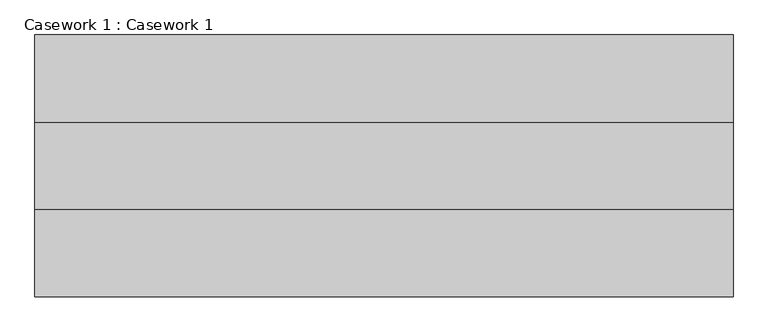
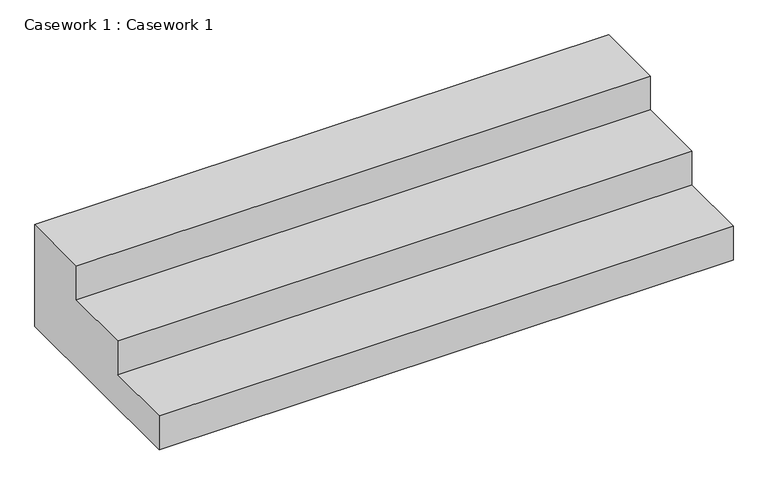
"""IFC4 building model written with IfcOpenShell, lengths in millimetres: furniture geometry, Casework 1 : Casework 1."""

from ifc_helpers import new_model, si_unit, frame, origin, place, context, project, spatial, polyline, outline, extrude, source, transform, mapped, element, save


def casework_1_casework_1_59e189ff(model_context):
    return source(origin(), model_context, "Body", "SweptSolid", [
        extrude(outline(polyline([(-6965.8839187, 1888.2737012), (-6661.0839187, 1888.2737012), (-6661.0839187, 1431.0737012), (-7575.4839187, 1431.0737012), (-7575.4839187, 1583.4737012), (-7270.6839187, 1583.4737012), (-7270.6839187, 1735.8737012), (-6965.8839187, 1735.8737012), (-6965.8839187, 1888.2737012)])), frame((-1552.5739162, 0.0, 0.0), z_axis=(1.0, 0.0, 0.0), x_axis=(0.0, 1.0, 0.0)), (0.0, 0.0, 1.0), 2438.4),
    ])


if __name__ == "__main__":
    model = new_model("IFC4")
    model_context = context("Model", 3, world=origin())
    ifc_project = project(units=[si_unit("LENGTHUNIT", "METRE", prefix="MILLI")], contexts=[model_context])
    site = spatial("IfcSite", under=ifc_project)
    building = spatial("IfcBuilding", under=site)
    placement = place(None, origin())
    casework_1_casework_1_shape = casework_1_casework_1_59e189ff(model_context)
    element("IfcFurniture", 1, ObjectType="Casework 1 : Casework 1", at=placement, inside=building, context=model_context, shape_type="MappedRepresentation", body=[
        mapped(casework_1_casework_1_shape, transform((0.0, 0.0, 0.0), x_axis=(1.0, 0.0, 0.0), y_axis=(0.0, 1.0, 0.0), z_axis=(0.0, 0.0, 1.0))),
    ])
    save(model, "model.ifc")
